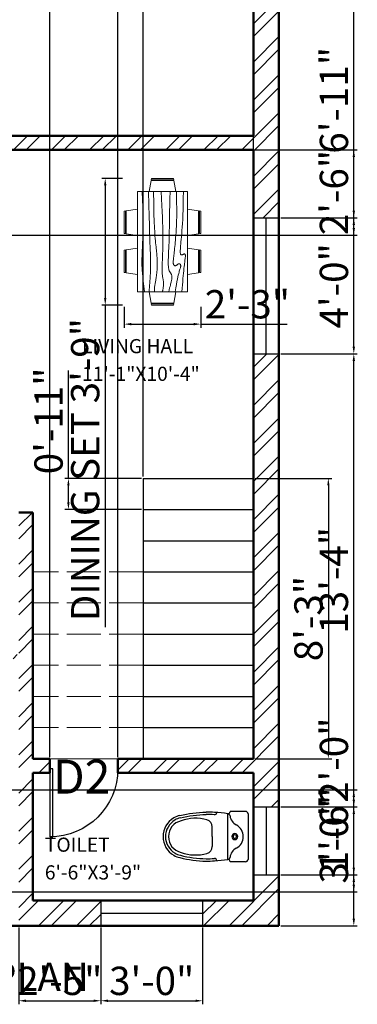
# Model space of a CAD drawing. Units: inches. Extents: x 3824 to 4289, y 1731 to 2259.
# Tile 4 of 5: x 4069 to 4188, y 1731 to 2079. Entities that reach past the tile are written whole.
import ezdxf

# ---------------------------------------------------------------- set-up
doc = ezdxf.new("R2010")
doc.units = ezdxf.units.IN
doc.linetypes.add('ACAD_ISO02W100', pattern=[15, 12, -3])
for name, color, linetype, lineweight in [('A-ANNO-DIMS', 2, 'Continuous', 18), ('A-ANNO-TEXT', 2, 'Continuous', 18), ('A-ANNO-TITL', 2, 'Continuous', 25), ('A-AREA-IDEN', 2, 'Continuous', 18), ('A-FLOR-FIXT', 9, 'Continuous', 18), ('A-FLOR-STRS-OVHD', 230, 'ACAD_ISO02W100', 18), ('A-FLOR-THRS', 8, 'Continuous', 18), ('A-FURN', 9, 'Continuous', 18), ('DOOR', 6, 'Continuous', 25), ('STAIRS', 230, 'Continuous', 25), ('WALL', 20, 'Continuous', 50), ('WINDOW', 4, 'Continuous', 25)]:
    doc.layers.add(name, color=color, linetype=linetype, lineweight=lineweight)
doc.layers.add('A-WALL-PATT', color=251, linetype='Continuous', lineweight=13, true_color=0x636466)
doc.layers.add('THIET-BI', color=21, linetype='Continuous')
doc.styles.get("Standard").update_dxf_attribs({"font": 'arial.ttf'})
doc.dimstyles.new('ISO-25', dxfattribs={"dimtxt": 10, "dimasz": 2.5, "dimexe": 1.25, "dimexo": 0.625, "dimtad": 1, "dimdec": 1, "dimlunit": 3, "dimtxsty": 'Standard', "dimcen": 2.5, "dimadec": 0, "dimazin": 0, "dimtfac": 1, "dimtdec": 1, "dimtmove": 0, "dimatfit": 3, "dimfxl": 1, "dimarcsym": 0})

# ---------------------------------------------------------------- blocks, each defined once
blk = doc.blocks.new('*U2')
for p, q in [((0, 0), (0, -6)), ((40, 0), (40, -6))]:
    blk.add_line(p, q)
blk.add_lwpolyline([(0, 0), (0, 40), (1.75, 40), (1.75, 0)], close=True)
blk.add_arc((0, 0), 40, 0, 90)
blk = doc.blocks.new('Dining Set - 36 x 72 in.')
for p, q in [((-22.2343, 26.00059), (-23.4847, 17.99762)), ((-22.2304, 26), (-5.7608, 26)), ((-22, 27.5), (-22.1562, 26.50042)), ((-5.8416, 26.5), (-22.1534, 26.5)), ((-22, 27.5), (-6, 27.5)), ((-5.8437, 26.49966), (-6, 27.5)), ((-4.5152, 17.99762), (-5.7655, 25.99926)), ((5.7657, 26.00059), (4.5153, 17.99762)), ((5.7696, 26), (22.2392, 26)), ((6, 27.5), (5.8438, 26.50042)), ((22.1584, 26.5), (5.8466, 26.5)), ((6, 27.5), (22, 27.5)), ((22.1563, 26.49966), (22, 27.5)), ((23.4848, 17.99762), (22.2345, 25.99926)), ((36, 18), (-36, 18)), ((-36, 18), (-36, -18)), ((36, -18), (36, 18)), ((-45.5, 8), (-44.5004, 8.15617)), ((-45.5, 8), (-45.5, -8)), ((-44.5, -8.15843), (-44.5, 8.15338)), ((-44.0006, 8.23428), (-35.9976, 9.48474)), ((-44, 8.23041), (-44, -8.23915)), ((44.0006, 8.23428), (35.9976, 9.48474)), ((44, 8.23041), (44, -8.23915)), ((44.5, -8.15843), (44.5, 8.15338)), ((45.5, 8), (44.5005, 8.15617)), ((45.5, 8), (45.5, -8)), ((-44.4997, -8.15631), (-45.5, -8)), ((-35.9976, -9.48476), (-43.9993, -8.2345)), ((35.9976, -9.48476), (43.9993, -8.2345)), ((44.4997, -8.15631), (45.5, -8)), ((-36, -18), (36, -18)), ((-22.2343, -26.0006), (-23.4847, -17.99762)), ((-4.5152, -17.99762), (-5.7655, -25.99928)), ((5.7657, -26.0006), (4.5153, -17.99762)), ((23.4848, -17.99762), (22.2345, -25.99928)), ((-22.2304, -26), (-5.7608, -26)), ((-22, -27.5), (-22.1562, -26.50044)), ((-5.8416, -26.5), (-22.1534, -26.5)), ((-22, -27.5), (-6, -27.5)), ((-5.8437, -26.49967), (-6, -27.5)), ((5.7696, -26), (22.2392, -26)), ((6, -27.5), (5.8438, -26.50044)), ((22.1584, -26.5), (5.8466, -26.5)), ((6, -27.5), (22, -27.5)), ((22.1563, -26.49967), (22, -27.5))]:
    blk.add_line(p, q)
for points in [[(-36, 15), (-31.1772, 14.97754), (-26.8079, 14.91406), (-22.8538, 14.81543), (-19.276, 14.6875), (-16.0362, 14.53613), (-13.0957, 14.36718), (-10.4159, 14.18652), (-7.9583, 14), (-5.6904, 13.81315), (-3.6035, 13.63021), (-1.6954, 13.45508), (0.0365, 13.29166), (1.5945, 13.14388), (2.9811, 13.01562), (4.1988, 12.9108), (5.25, 12.83333), (6.1393, 12.78613), (6.8802, 12.76823), (7.4883, 12.77767), (7.9792, 12.8125), (8.3685, 12.87077), (8.6719, 12.95052), (8.9049, 13.0498), (9.0833, 13.16666), (9.2205, 13.29899), (9.3216, 13.44401), (9.3895, 13.59879), (9.4271, 13.76041), (9.4373, 13.92594), (9.4232, 14.09245), (9.3875, 14.257), (9.3333, 14.41666), (9.2638, 14.56917), (9.1836, 14.71484), (9.0975, 14.85465), (9.0104, 14.98958), (8.9272, 15.1206), (8.8529, 15.2487), (8.7922, 15.37483), (8.75, 15.5), (8.7305, 15.62467), (8.7344, 15.74739), (8.7617, 15.86621), (8.8125, 15.97916), (8.8867, 16.08431), (8.9844, 16.17968), (9.1055, 16.26334), (9.25, 16.33333), (9.4189, 16.38802), (9.6172, 16.42708), (9.8506, 16.45052), (10.125, 16.45833), (10.4463, 16.45052), (10.8203, 16.42708), (11.2529, 16.38802), (11.75, 16.33333), (12.3184, 16.26318), (12.9694, 16.17838), (13.7151, 16.07991), (14.5677, 15.96875), (15.5395, 15.84586), (16.6426, 15.71224), (17.8893, 15.56884), (19.2917, 15.41666), (20.859, 15.25667), (22.5879, 15.08984), (24.4721, 14.91715), (26.5052, 14.73958), (28.6809, 14.5581), (30.9929, 14.3737), (33.4347, 14.18733), (36, 14)], [(-36, 10), (-28.9766, 10.14274), (-23.1725, 10.20442), (-18.4241, 10.19775), (-14.5677, 10.13541), (-11.4399, 10.03011), (-8.877, 9.89453), (-6.7154, 9.74137), (-4.7917, 9.58333), (-2.9698, 9.43082), (-1.2246, 9.28515), (0.4415, 9.14534), (2.026, 9.01041), (3.5266, 8.87939), (4.9408, 8.7513), (6.266, 8.62516), (7.5, 8.5), (8.6411, 8.37549), (9.6914, 8.2539), (10.6538, 8.13818), (11.5312, 8.03125), (12.3267, 7.93603), (13.043, 7.85547), (13.6831, 7.79248), (14.25, 7.75), (14.7471, 7.7303), (15.1797, 7.73307), (15.5537, 7.75732), (15.875, 7.80208), (16.1494, 7.86637), (16.3828, 7.94922), (16.5811, 8.04964), (16.75, 8.16666), (16.8944, 8.29915), (17.0143, 8.44531), (17.1089, 8.60319), (17.1771, 8.77083), (17.218, 8.94629), (17.2305, 9.1276), (17.2137, 9.31282), (17.1667, 9.5), (17.0895, 9.6875), (16.987, 9.875), (16.8649, 10.0625), (16.7292, 10.25), (16.5856, 10.4375), (16.4401, 10.625), (16.2985, 10.8125), (16.1667, 11), (16.05, 11.18733), (15.9518, 11.3737), (15.8752, 11.5581), (15.8229, 11.73958), (15.798, 11.91715), (15.8034, 12.08984), (15.842, 12.25667), (15.9167, 12.41666), (16.0295, 12.56836), (16.1784, 12.70833), (16.3605, 12.83268), (16.5729, 12.9375), (16.8127, 13.01888), (17.0768, 13.07291), (17.3625, 13.0957), (17.6667, 13.08333), (17.9894, 13.03312), (18.3418, 12.94726), (18.7382, 12.82918), (19.1927, 12.68229), (19.7195, 12.51001), (20.3327, 12.31575), (21.0465, 12.10294), (21.875, 11.875), (22.8357, 11.63354), (23.959, 11.37304), (25.2786, 11.08618), (26.8282, 10.76562), (28.6414, 10.40405), (30.752, 9.99414), (33.1936, 9.52856), (36, 9)], [(-36, 5.5), (-30.7157, 5.3348), (-26.069, 5.20963), (-21.9946, 5.11767), (-18.4271, 5.05208), (-15.3009, 5.00602), (-12.5508, 4.97265), (-10.1112, 4.94515), (-7.9167, 4.91666), (-5.909, 4.88167), (-4.0586, 4.83984), (-2.3429, 4.79215), (-0.7396, 4.73958), (0.7739, 4.6831), (2.22, 4.6237), (3.6213, 4.56233), (5, 4.5), (6.373, 4.43782), (7.7344, 4.3776), (9.0723, 4.32129), (10.375, 4.27083), (11.6309, 4.22819), (12.8281, 4.19531), (13.9551, 4.17415), (15, 4.16666), (15.954, 4.17448), (16.819, 4.19791), (17.6001, 4.23698), (18.3021, 4.29166), (18.9299, 4.36198), (19.4883, 4.44791), (19.9823, 4.54948), (20.4167, 4.66666), (20.7969, 4.79899), (21.1302, 4.94401), (21.4245, 5.09879), (21.6875, 5.26041), (21.9271, 5.42594), (22.1511, 5.59245), (22.3672, 5.757), (22.5834, 5.91666), (22.8065, 6.06868), (23.0404, 6.21093), (23.2879, 6.34147), (23.5521, 6.45833), (23.8358, 6.55957), (24.142, 6.64323), (24.4735, 6.70735), (24.8334, 6.75), (25.2235, 6.76969), (25.642, 6.76692), (26.0858, 6.74267), (26.5521, 6.69791), (27.0379, 6.63362), (27.5404, 6.55078), (28.0565, 6.45036), (28.5834, 6.33333), (29.1242, 6.19987), (29.7071, 6.04687), (30.3661, 5.87044), (31.1354, 5.66666), (32.0493, 5.43164), (33.142, 5.16146), (34.4475, 4.85221), (36, 4.5)], [(-36, -1), (-30.7915, -0.6591), (-26.0195, -0.38216), (-21.6519, -0.16284), (-17.6563, 0.00521), (-14.0005, 0.12833), (-10.6523, 0.21289), (-7.5796, 0.26522), (-4.75, 0.29166), (-2.134, 0.29793), (0.2878, 0.28711), (2.5317, 0.26163), (4.6146, 0.22396), (6.5529, 0.17651), (8.3633, 0.12174), (10.0623, 0.06209), (11.6667, 0), (13.1899, -0.06201), (14.6341, -0.1211), (15.9982, -0.17432), (17.2813, -0.21875), (18.4823, -0.25147), (19.6003, -0.26953), (20.6343, -0.27002), (21.5834, -0.25), (22.4481, -0.20768), (23.2357, -0.14584), (23.9549, -0.06836), (24.6146, 0.02083), (25.2235, 0.11784), (25.7904, 0.21875), (26.3241, 0.31966), (26.8334, 0.41666), (27.3265, 0.50618), (27.8099, 0.58593), (28.2894, 0.65397), (28.7709, 0.70833), (29.2601, 0.74707), (29.763, 0.76823), (30.2855, 0.76985), (30.8334, 0.75), (31.4088, 0.70784), (31.9994, 0.64713), (32.589, 0.57275), (33.1615, 0.48958), (33.7008, 0.4025), (34.1908, 0.3164), (34.6153, 0.23616), (34.9584, 0.16666), (35.2099, 0.11165), (35.3848, 0.07031), (35.504, 0.04069), (35.5886, 0.02083), (35.6594, 0.00879), (35.7377, 0.0026), (35.8442, 0.00032), (36, 0)], [(-36, -6.5), (-27.1843, -6.31267), (-20.084, -6.1263), (-14.469, -5.9419), (-10.1094, -5.76042), (-6.7752, -5.58285), (-4.2363, -5.41016), (-2.2629, -5.24333), (-0.625, -5.08334), (0.8708, -4.93099), (2.2715, -4.78646), (3.5872, -4.64974), (4.8281, -4.52084), (6.0046, -4.39974), (7.127, -4.28646), (8.2053, -4.18099), (9.25, -4.08334), (10.2705, -3.99382), (11.2734, -3.91407), (12.2647, -3.84603), (13.25, -3.79167), (14.2354, -3.75293), (15.2266, -3.73177), (16.2295, -3.73015), (17.25, -3.75), (18.2912, -3.79248), (19.3451, -3.85547), (20.4009, -3.93604), (21.4479, -4.03125), (22.4754, -4.13819), (23.4727, -4.25391), (24.4289, -4.37549), (25.3334, -4.5), (26.1785, -4.62492), (26.9694, -4.74935), (27.7145, -4.87281), (28.4219, -4.99479), (29.1, -5.11483), (29.7572, -5.23242), (30.4016, -5.34709), (31.0417, -5.45834), (31.6837, -5.56437), (32.3262, -5.65821), (32.9658, -5.73153), (33.599, -5.77604), (34.2224, -5.78345), (34.8327, -5.74545), (35.4264, -5.65373), (36, -5.5)], [(-36, -10), (-26.4022, -9.81299), (-18.4675, -9.62891), (-11.9839, -9.45069), (-6.7396, -9.28125), (-2.5226, -9.12354), (0.8789, -8.98047), (3.6769, -8.85498), (6.0833, -8.75), (8.2767, -8.66765), (10.3021, -8.60677), (12.1712, -8.56543), (13.8958, -8.54167), (15.4876, -8.53353), (16.9583, -8.53907), (18.3197, -8.55632), (19.5834, -8.58334), (20.7616, -8.61841), (21.8685, -8.66081), (22.9188, -8.71004), (23.9271, -8.76563), (24.9081, -8.82707), (25.8763, -8.89388), (26.8465, -8.96558), (27.8334, -9.04167), (28.8474, -9.12118), (29.8828, -9.20117), (30.93, -9.27824), (31.9792, -9.34896), (33.0205, -9.40991), (34.0443, -9.45768), (35.0407, -9.48885), (36, -9.5)], [(-36, -14.5), (-30.0881, -14.33513), (-25.0332, -14.21224), (-20.7312, -14.12647), (-17.0781, -14.07292), (-13.97, -14.04671), (-11.3027, -14.04297), (-8.9724, -14.05681), (-6.875, -14.08334), (-4.9224, -14.11833), (-3.0905, -14.16016), (-1.3709, -14.20785), (0.2448, -14.26042), (1.7647, -14.3169), (3.1973, -14.3763), (4.5507, -14.43767), (5.8333, -14.5), (7.0554, -14.5621), (8.235, -14.62175), (9.3922, -14.67652), (10.5469, -14.72396), (11.7192, -14.76164), (12.929, -14.78711), (14.1965, -14.79794), (15.5417, -14.79167), (16.9933, -14.76424), (18.6152, -14.70508), (20.4804, -14.60197), (22.6615, -14.44271), (25.2312, -14.21509), (28.2624, -13.9069), (31.8277, -13.50594), (36, -13)]]:
    blk.add_lwpolyline(points)
blk = doc.blocks.new('A$C7C314EA1')
at = {"layer": 'THIET-BI'}
for p, q in [((20, 420), (150, 420)), ((0, 20), (0, 400)), ((170, 400), (170, 20)), ((300, 210), (300, 292.2)), ((300, 210), (300, 127.8)), ((20, 0), (150, 0)), ((20, 0), (150, 0))]:
    blk.add_line(p, q, dxfattribs=at)
for points in [[(279.9, 412.5, 0.02753), (170, 400, 0.02753)], [(569.7, 385.6, 0.054905), (350, 415, 0.054905)], [(564.9, 366.1, 0.054905), (349.5, 395, 0.054905)], [(300, 210), (300, 290, 0.704392)], [(300, 210), (300, 130, -0.704392)], [(170, 20, 0.02753), (279.9, 7.5, 0.02753)], [(564.9, 53.9, -0.054905), (349.5, 25, -0.054905)], [(569.7, 34.4, -0.054905), (350, 5, -0.054905)]]:
    blk.add_lwpolyline(points, format="xyb", dxfattribs=at)
for centre, radius, start, end in [((20, 400), 20, 90, 180), ((170, 420), 20, 180, 270), ((279.9, 412.5), 20, 184.59048, 273.88227), ((350, -585), 1000, 90, 94.02044), ((51, 395.2), 100, 298.13818, 352.73228), ((170, 380), 20, 90, 172.73228), ((350, -585), 980, 90, 94.02044), ((360, 292.2), 60, 105.92494, 180), ((439, 15.2), 348.1, 69.70099, 105.92494), ((530, 210), 135, 0, 77.24247), ((530, 210), 160, 60, 77.24247), ((530, 210), 180, 60, 77.24247), ((530, 210), 160, 0, 60), ((530, 210), 180, 0, 60), ((150, 210), 110, 118.13818, 180), ((150, 210), 110, 180, 241.86182), ((150, 210), 110, 180, 241.86182), ((110, 210), 25, 0, 180), ((110, 210), 25, 0, 180), ((110, 210), 25, 180, 0), ((110, 210), 25, 180, 0), ((110, 210), 15, 0, 180), ((110, 210), 15, 0, 180), ((110, 210), 15, 180, 0), ((110, 210), 15, 180, 0), ((530, 210), 135, 282.75753, 0), ((530, 210), 160, 300, 0), ((530, 210), 180, 300, 0), ((51, 24.8), 100, 7.26772, 61.86182), ((51, 24.8), 100, 7.26772, 61.86182), ((360, 127.8), 60, 180, 254.07506), ((20, 20), 20, 180, 270), ((170, 0), 20, 90, 180), ((170, 40), 20, 187.26772, 270), ((170, 40), 20, 187.26772, 270), ((279.9, 7.5), 20, 86.11773, 175.40952), ((350, 1005), 1000, 265.97956, 270), ((350, 1005), 980, 265.97956, 270), ((439, 404.8), 348.1, 254.07506, 290.29901), ((530, 210), 160, 282.75753, 300), ((530, 210), 180, 282.75753, 300)]:
    blk.add_arc(centre, radius, start, end, dxfattribs=at)
blk = doc.blocks.new('*D20')
at = {"layer": 'A-ANNO-DIMS', "color": 0, "lineweight": -2, "transparency": 16777216}
for p, q in [((4105.21, 2022.56), (4097.87, 2022.56)), ((4099.12, 2020.06), (4099.12, 1980.29)), ((4105.21, 1977.79), (4097.87, 1977.79)), ((4099.12, 1977.79), (4099.12, 1864.13))]:
    blk.add_line(p, q, dxfattribs=at)
at = {"layer": 'A-ANNO-DIMS', "color": 0, "transparency": 16777216}
for points in [[(4098.7, 2020.06), (4099.53, 2020.06), (4099.12, 2022.56)], [(4098.7, 1980.29), (4099.53, 1980.29), (4099.12, 1977.79)]]:
    blk.add_solid(points, dxfattribs=at)
at = {"layer": 'Defpoints', "color": 0, "transparency": 16777216}
for p in [(4105.83, 2022.56), (4099.12, 1977.79), (4105.83, 1977.79)]:
    blk.add_point(p, dxfattribs=at)
at = {"layer": 'A-ANNO-DIMS', "color": 0, "transparency": 16777216, "insert": (4093.32, 1919.71), "char_height": 10, "attachment_point": 5, "rotation": 90}
blk.add_mtext('DINING SET 3\'-9"', dxfattribs=at)
blk = doc.blocks.new('*D21')
at = {"layer": 'A-ANNO-DIMS', "color": 0, "lineweight": -2, "transparency": 16777216}
for p, q in [((4105.83, 1977.17), (4105.83, 1969.83)), ((4132.89, 1977.17), (4132.89, 1969.83)), ((4108.33, 1971.08), (4130.39, 1971.08)), ((4132.89, 1971.08), (4163.39, 1971.08))]:
    blk.add_line(p, q, dxfattribs=at)
at = {"layer": 'A-ANNO-DIMS', "color": 0, "transparency": 16777216}
for points in [[(4108.33, 1971.5), (4108.33, 1970.66), (4105.83, 1971.08)], [(4130.39, 1971.5), (4130.39, 1970.66), (4132.89, 1971.08)]]:
    blk.add_solid(points, dxfattribs=at)
at = {"layer": 'Defpoints', "color": 0, "transparency": 16777216}
for p in [(4105.83, 1977.79), (4132.89, 1977.79), (4132.89, 1971.08)]:
    blk.add_point(p, dxfattribs=at)
at = {"layer": 'A-ANNO-DIMS', "color": 0, "transparency": 16777216, "insert": (4149.39, 1976.81), "char_height": 10, "attachment_point": 5}
blk.add_mtext('2\'-3"', dxfattribs=at)
blk = doc.blocks.new('*D32')
at = {"layer": 'A-ANNO-DIMS', "color": 0, "lineweight": -2, "transparency": 16777216}
for p, q in [((4187, 1776.62), (4187, 1806.01)), ((4161.18, 1776.62), (4188.25, 1776.62)), ((4187, 1761.12), (4187, 1774.12)), ((4161.18, 1758.62), (4188.25, 1758.62))]:
    blk.add_line(p, q, dxfattribs=at)
at = {"layer": 'A-ANNO-DIMS', "color": 0, "transparency": 16777216}
for points in [[(4186.59, 1774.12), (4187.42, 1774.12), (4187, 1776.62)], [(4186.59, 1761.12), (4187.42, 1761.12), (4187, 1758.62)]]:
    blk.add_solid(points, dxfattribs=at)
at = {"layer": 'Defpoints', "color": 0, "transparency": 16777216}
for p in [(4160.55, 1776.62), (4187, 1776.62), (4160.55, 1758.62)]:
    blk.add_point(p, dxfattribs=at)
at = {"layer": 'A-ANNO-DIMS', "color": 0, "transparency": 16777216, "insert": (4181.27, 1792.56), "char_height": 10, "attachment_point": 5, "rotation": 90}
blk.add_mtext('1\'-6"', dxfattribs=at)
blk = doc.blocks.new('*D33')
at = {"layer": 'A-ANNO-DIMS', "color": 0, "lineweight": -2, "transparency": 16777216}
for p, q in [((4187, 1800.62), (4187, 1831.12)), ((4161.18, 1800.62), (4188.25, 1800.62)), ((4187, 1779.12), (4187, 1798.12)), ((4161.18, 1776.62), (4188.25, 1776.62))]:
    blk.add_line(p, q, dxfattribs=at)
at = {"layer": 'A-ANNO-DIMS', "color": 0, "transparency": 16777216}
for points in [[(4186.59, 1798.12), (4187.42, 1798.12), (4187, 1800.62)], [(4186.59, 1779.12), (4187.42, 1779.12), (4187, 1776.62)]]:
    blk.add_solid(points, dxfattribs=at)
at = {"layer": 'Defpoints', "color": 0, "transparency": 16777216}
for p in [(4160.55, 1800.62), (4187, 1800.62), (4160.55, 1776.62)]:
    blk.add_point(p, dxfattribs=at)
at = {"layer": 'A-ANNO-DIMS', "color": 0, "transparency": 16777216, "insert": (4181.27, 1817.12), "char_height": 10, "attachment_point": 5, "rotation": 90}
blk.add_mtext('2\'-0"', dxfattribs=at)
blk = doc.blocks.new('*D34')
at = {"layer": 'A-ANNO-DIMS', "color": 0, "lineweight": -2, "transparency": 16777216}
for p, q in [((4161.18, 1960.62), (4188.25, 1960.62)), ((4187, 1803.12), (4187, 1958.12)), ((4161.18, 1800.62), (4188.25, 1800.62))]:
    blk.add_line(p, q, dxfattribs=at)
at = {"layer": 'A-ANNO-DIMS', "color": 0, "transparency": 16777216}
for points in [[(4186.59, 1958.12), (4187.42, 1958.12), (4187, 1960.62)], [(4186.59, 1803.12), (4187.42, 1803.12), (4187, 1800.62)]]:
    blk.add_solid(points, dxfattribs=at)
at = {"layer": 'Defpoints', "color": 0, "transparency": 16777216}
for p in [(4160.55, 1960.62), (4187, 1960.62), (4160.55, 1800.62)]:
    blk.add_point(p, dxfattribs=at)
at = {"layer": 'A-ANNO-DIMS', "color": 0, "transparency": 16777216, "insert": (4181.27, 1880.62), "char_height": 10, "attachment_point": 5, "rotation": 90}
blk.add_mtext('13\'-4"', dxfattribs=at)
blk = doc.blocks.new('*D35')
at = {"layer": 'A-ANNO-DIMS', "color": 0, "lineweight": -2, "transparency": 16777216}
for p, q in [((4161.18, 2008.62), (4188.25, 2008.62)), ((4187, 1963.12), (4187, 2006.12)), ((4161.18, 1960.62), (4188.25, 1960.62))]:
    blk.add_line(p, q, dxfattribs=at)
at = {"layer": 'A-ANNO-DIMS', "color": 0, "transparency": 16777216}
for points in [[(4186.59, 2006.12), (4187.42, 2006.12), (4187, 2008.62)], [(4186.59, 1963.12), (4187.42, 1963.12), (4187, 1960.62)]]:
    blk.add_solid(points, dxfattribs=at)
at = {"layer": 'Defpoints', "color": 0, "transparency": 16777216}
for p in [(4160.55, 2008.62), (4187, 2008.62), (4160.55, 1960.62)]:
    blk.add_point(p, dxfattribs=at)
at = {"layer": 'A-ANNO-DIMS', "color": 0, "transparency": 16777216, "insert": (4181.27, 1984.62), "char_height": 10, "attachment_point": 5, "rotation": 90}
blk.add_mtext('4\'-0"', dxfattribs=at)
blk = doc.blocks.new('*D36')
at = {"layer": 'A-ANNO-DIMS', "color": 0, "lineweight": -2, "transparency": 16777216}
for p, q in [((4161.18, 2091.62), (4188.25, 2091.62)), ((4187, 2011.12), (4187, 2089.12)), ((4161.18, 2008.62), (4188.25, 2008.62))]:
    blk.add_line(p, q, dxfattribs=at)
at = {"layer": 'A-ANNO-DIMS', "color": 0, "transparency": 16777216}
for points in [[(4186.59, 2089.12), (4187.42, 2089.12), (4187, 2091.62)], [(4186.59, 2011.12), (4187.42, 2011.12), (4187, 2008.62)]]:
    blk.add_solid(points, dxfattribs=at)
at = {"layer": 'Defpoints', "color": 0, "transparency": 16777216}
for p in [(4160.55, 2091.62), (4187, 2091.62), (4160.55, 2008.62)]:
    blk.add_point(p, dxfattribs=at)
at = {"layer": 'A-ANNO-DIMS', "color": 0, "transparency": 16777216, "insert": (4181.27, 2050.12), "char_height": 10, "attachment_point": 5, "rotation": 90}
blk.add_mtext('6\'-11"', dxfattribs=at)
blk = doc.blocks.new('*D40')
at = {"layer": 'A-ANNO-DIMS', "color": 0, "lineweight": -2, "transparency": 16777216}
for p, q in [((4068.55, 1757.99), (4068.55, 1730.92)), ((4097.55, 1757.99), (4097.55, 1730.92)), ((4071.05, 1732.17), (4095.05, 1732.17))]:
    blk.add_line(p, q, dxfattribs=at)
at = {"layer": 'A-ANNO-DIMS', "color": 0, "transparency": 16777216}
for points in [[(4071.05, 1732.59), (4071.05, 1731.75), (4068.55, 1732.17)], [(4095.05, 1732.59), (4095.05, 1731.75), (4097.55, 1732.17)]]:
    blk.add_solid(points, dxfattribs=at)
at = {"layer": 'Defpoints', "color": 0, "transparency": 16777216}
for p in [(4068.55, 1758.62), (4097.55, 1758.62), (4097.55, 1732.17)]:
    blk.add_point(p, dxfattribs=at)
at = {"layer": 'A-ANNO-DIMS', "color": 0, "transparency": 16777216, "insert": (4083.05, 1737.9), "char_height": 10, "attachment_point": 5}
blk.add_mtext('2\'-5"', dxfattribs=at)
blk = doc.blocks.new('*D41')
at = {"layer": 'A-ANNO-DIMS', "color": 0, "lineweight": -2, "transparency": 16777216}
for p, q in [((4097.55, 1757.99), (4097.55, 1730.92)), ((4133.55, 1757.99), (4133.55, 1730.92)), ((4100.05, 1732.17), (4131.05, 1732.17))]:
    blk.add_line(p, q, dxfattribs=at)
at = {"layer": 'A-ANNO-DIMS', "color": 0, "transparency": 16777216}
for points in [[(4100.05, 1732.59), (4100.05, 1731.75), (4097.55, 1732.17)], [(4131.05, 1732.59), (4131.05, 1731.75), (4133.55, 1732.17)]]:
    blk.add_solid(points, dxfattribs=at)
at = {"layer": 'Defpoints', "color": 0, "transparency": 16777216}
for p in [(4097.55, 1758.62), (4133.55, 1758.62), (4133.55, 1732.17)]:
    blk.add_point(p, dxfattribs=at)
at = {"layer": 'A-ANNO-DIMS', "color": 0, "transparency": 16777216, "insert": (4115.55, 1737.9), "char_height": 10, "attachment_point": 5}
blk.add_mtext('3\'-0"', dxfattribs=at)
blk = doc.blocks.new('*D49')
at = {"layer": 'A-ANNO-DIMS', "color": 0, "lineweight": -2, "transparency": 16777216}
for p, q in [((3965.18, 1806.62), (4188.25, 1806.62)), ((4187, 1773.12), (4187, 1804.12)), ((3965.18, 1770.62), (4188.25, 1770.62))]:
    blk.add_line(p, q, dxfattribs=at)
at = {"layer": 'A-ANNO-DIMS', "color": 0, "transparency": 16777216}
for points in [[(4186.59, 1804.12), (4187.42, 1804.12), (4187, 1806.62)], [(4186.59, 1773.12), (4187.42, 1773.12), (4187, 1770.62)]]:
    blk.add_solid(points, dxfattribs=at)
at = {"layer": 'Defpoints', "color": 0, "transparency": 16777216}
for p in [(3964.55, 1806.62), (4187, 1806.62), (3964.55, 1770.62)]:
    blk.add_point(p, dxfattribs=at)
at = {"layer": 'A-ANNO-DIMS', "color": 0, "transparency": 16777216, "insert": (4181.27, 1788.62), "char_height": 10, "attachment_point": 5, "rotation": 90}
blk.add_mtext('3\'-0"', dxfattribs=at)
blk = doc.blocks.new('*D50')
at = {"layer": 'A-ANNO-DIMS', "color": 0, "lineweight": -2, "transparency": 16777216}
for p, q in [((4079.55, 1818.24), (4079.55, 2230.32)), ((4082.05, 2229.07), (4101.05, 2229.07)), ((4103.55, 1818.24), (4103.55, 2230.32)), ((4103.55, 2229.07), (4134.06, 2229.07))]:
    blk.add_line(p, q, dxfattribs=at)
at = {"layer": 'A-ANNO-DIMS', "color": 0, "transparency": 16777216}
for points in [[(4082.05, 2229.49), (4082.05, 2228.65), (4079.55, 2229.07)], [(4101.05, 2229.49), (4101.05, 2228.65), (4103.55, 2229.07)]]:
    blk.add_solid(points, dxfattribs=at)
at = {"layer": 'Defpoints', "color": 0, "transparency": 16777216}
for p in [(4103.55, 2229.07), (4079.55, 1817.62), (4103.55, 1817.62)]:
    blk.add_point(p, dxfattribs=at)
at = {"layer": 'A-ANNO-DIMS', "color": 0, "transparency": 16777216, "insert": (4120.05, 2234.8), "char_height": 10, "attachment_point": 5}
blk.add_mtext('2\'-0"', dxfattribs=at)
blk = doc.blocks.new('*D51')
at = {"layer": 'A-ANNO-DIMS', "color": 0, "lineweight": -2, "transparency": 16777216}
for p, q in [((4112.55, 1917.24), (4112.55, 2230.32)), ((4115.05, 2229.07), (4149.05, 2229.07)), ((4151.55, 1917.24), (4151.55, 2230.32))]:
    blk.add_line(p, q, dxfattribs=at)
at = {"layer": 'A-ANNO-DIMS', "color": 0, "transparency": 16777216}
for points in [[(4115.05, 2229.49), (4115.05, 2228.65), (4112.55, 2229.07)], [(4149.05, 2229.49), (4149.05, 2228.65), (4151.55, 2229.07)]]:
    blk.add_solid(points, dxfattribs=at)
at = {"layer": 'Defpoints', "color": 0, "transparency": 16777216}
for p in [(4151.55, 2229.07), (4112.55, 1916.62), (4151.55, 1916.62)]:
    blk.add_point(p, dxfattribs=at)
at = {"layer": 'A-ANNO-DIMS', "color": 0, "transparency": 16777216, "insert": (4132.05, 2234.8), "char_height": 10, "attachment_point": 5}
blk.add_mtext('3\'-3"', dxfattribs=at)
blk = doc.blocks.new('*D52')
at = {"layer": 'A-ANNO-DIMS', "color": 0, "lineweight": -2, "transparency": 16777216}
for p, q in [((4152.18, 1916.62), (4179.25, 1916.62)), ((4178, 1914.12), (4178, 1820.12)), ((4152.18, 1817.62), (4179.25, 1817.62))]:
    blk.add_line(p, q, dxfattribs=at)
at = {"layer": 'A-ANNO-DIMS', "color": 0, "transparency": 16777216}
for points in [[(4177.59, 1914.12), (4178.42, 1914.12), (4178, 1916.62)], [(4177.59, 1820.12), (4178.42, 1820.12), (4178, 1817.62)]]:
    blk.add_solid(points, dxfattribs=at)
at = {"layer": 'Defpoints', "color": 0, "transparency": 16777216}
for p in [(4151.55, 1916.62), (4151.55, 1817.62), (4178, 1817.62)]:
    blk.add_point(p, dxfattribs=at)
at = {"layer": 'A-ANNO-DIMS', "color": 0, "transparency": 16777216, "insert": (4172.27, 1867.12), "char_height": 10, "attachment_point": 5, "rotation": 90}
blk.add_mtext('8\'-3"', dxfattribs=at)
blk = doc.blocks.new('*D53')
at = {"layer": 'A-ANNO-DIMS', "color": 0, "lineweight": -2, "transparency": 16777216}
for p, q in [((4086.1, 1916.62), (4086.1, 1954.72)), ((4111.93, 1916.62), (4084.85, 1916.62)), ((4086.1, 1908.12), (4086.1, 1914.12)), ((4111.93, 1905.62), (4084.85, 1905.62))]:
    blk.add_line(p, q, dxfattribs=at)
at = {"layer": 'A-ANNO-DIMS', "color": 0, "transparency": 16777216}
for points in [[(4085.69, 1914.12), (4086.52, 1914.12), (4086.1, 1916.62)], [(4085.69, 1908.12), (4086.52, 1908.12), (4086.1, 1905.62)]]:
    blk.add_solid(points, dxfattribs=at)
at = {"layer": 'Defpoints', "color": 0, "transparency": 16777216}
for p in [(4086.1, 1916.62), (4112.55, 1916.62), (4112.55, 1905.62)]:
    blk.add_point(p, dxfattribs=at)
at = {"layer": 'A-ANNO-DIMS', "color": 0, "transparency": 16777216, "insert": (4080.37, 1936.92), "char_height": 10, "attachment_point": 5, "rotation": 90}
blk.add_mtext('0\'-11"', dxfattribs=at)
blk = doc.blocks.new('*D62')
at = {"layer": 'A-ANNO-DIMS', "color": 0, "lineweight": -2, "transparency": 16777216}
for p, q in [((3898.51, 2032.62), (4188.25, 2032.62)), ((4187, 2005), (4187, 2030.12)), ((3898.51, 2002.5), (4188.25, 2002.5))]:
    blk.add_line(p, q, dxfattribs=at)
at = {"layer": 'A-ANNO-DIMS', "color": 0, "transparency": 16777216}
for points in [[(4186.59, 2030.12), (4187.42, 2030.12), (4187, 2032.62)], [(4186.59, 2005), (4187.42, 2005), (4187, 2002.5)]]:
    blk.add_solid(points, dxfattribs=at)
at = {"layer": 'Defpoints', "color": 0, "transparency": 16777216}
for p in [(3897.89, 2032.62), (4187, 2032.62), (3897.89, 2002.5)]:
    blk.add_point(p, dxfattribs=at)
at = {"layer": 'A-ANNO-DIMS', "color": 0, "transparency": 16777216, "insert": (4181.27, 2017.56), "char_height": 10, "attachment_point": 5, "rotation": 90}
blk.add_mtext('2\'-6"', dxfattribs=at)

msp = doc.modelspace()

# ---------------------------------------------------------------- hatches: boundary and pattern name
at = {"layer": 'A-WALL-PATT'}
h = msp.add_hatch(dxfattribs=at)
h.set_pattern_fill('ANSI32', color=256)
h.paths.add_polyline_path([(4160.55, 2091.62), (4151.55, 2091.62), (4151.55, 2037.62), (4063.55, 2037.62), (4063.55, 2032.62), (4151.55, 2032.62), (4151.55, 2008.62), (4160.55, 2008.62)])
h = msp.add_hatch(dxfattribs=at)
h.set_pattern_fill('ANSI32', color=256)
h.paths.add_polyline_path([(4160.55, 1960.62), (4151.55, 1960.62), (4151.55, 1817.62), (4103.55, 1817.62), (4103.55, 1814.02), (4103.55, 1812.62), (4151.55, 1812.62), (4151.55, 1800.62), (4160.55, 1800.62)])
h = msp.add_hatch(dxfattribs=at)
h.set_pattern_fill('ANSI32', color=256)
h.paths.add_polyline_path([(4073.55, 1904.62), (4068.55, 1904.62), (4068.55, 1854.39), (4066.55, 1854.39), (4066.55, 1849.39), (4068.55, 1849.39), (4068.55, 1767.62), (4068.55, 1758.62), (4097.55, 1758.62), (4097.55, 1767.62), (4073.55, 1767.62), (4073.55, 1812.62), (4079.55, 1812.62), (4079.55, 1817.62), (4073.55, 1817.62)])
h = msp.add_hatch(dxfattribs=at)
h.set_pattern_fill('ANSI32', color=256)
h.paths.add_polyline_path([(4160.55, 1776.62), (4151.55, 1776.62), (4151.55, 1767.62), (4133.55, 1767.62), (4133.55, 1758.62), (4160.55, 1758.62)])

# ---------------------------------------------------------------- linework, layer by layer
at = {"layer": 'A-FLOR-STRS-OVHD'}
for p, q in [((4112.55, 1883.62), (4073.55, 1883.62)), ((4112.55, 1872.62), (4073.55, 1872.62)), ((4112.55, 1861.62), (4073.55, 1861.62)), ((4112.55, 1850.62), (4073.55, 1850.62)), ((4112.55, 1839.62), (4073.55, 1839.62)), ((4112.55, 1828.62), (4073.55, 1828.62))]:
    msp.add_line(p, q, dxfattribs=at)
at = {"layer": 'A-FLOR-THRS'}
msp.add_line((4079.55, 1817.62), (4103.55, 1817.62), dxfattribs=at)
at = {"layer": 'STAIRS'}
for p, q in [((4112.55, 1916.62), (4151.55, 1916.62)), ((4112.55, 1916.62), (4112.55, 1817.62)), ((4112.55, 1905.62), (4151.55, 1905.62)), ((4112.55, 1894.62), (4151.55, 1894.62)), ((4112.55, 1883.62), (4151.55, 1883.62)), ((4112.55, 1872.62), (4151.55, 1872.62)), ((4112.55, 1861.62), (4151.55, 1861.62)), ((4112.55, 1850.62), (4151.55, 1850.62)), ((4112.55, 1839.62), (4151.55, 1839.62)), ((4112.55, 1828.62), (4151.55, 1828.62))]:
    msp.add_line(p, q, dxfattribs=at)
at = {"layer": 'WALL'}
for p, q in [((4160.55, 2202.62), (4160.55, 1758.62)), ((4151.55, 2193.62), (4151.55, 2037.62)), ((4063.55, 2037.62), (4151.55, 2037.62)), ((4063.55, 2032.62), (4151.55, 2032.62)), ((4151.55, 2032.62), (4151.55, 1817.62)), ((4068.55, 1904.62), (4073.55, 1904.62)), ((4073.55, 1904.62), (4073.55, 1817.62)), ((4073.55, 1817.62), (4079.55, 1817.62)), ((4079.55, 1817.62), (4079.55, 1812.62)), ((4103.55, 1817.62), (4103.55, 1812.62)), ((4103.55, 1817.62), (4151.55, 1817.62)), ((4073.55, 1812.62), (4079.55, 1812.62)), ((4073.55, 1812.62), (4073.55, 1767.62)), ((4103.55, 1812.62), (4151.55, 1812.62)), ((4151.55, 1812.62), (4151.55, 1767.62)), ((4073.55, 1767.62), (4151.55, 1767.62)), ((4013.55, 1758.62), (4160.55, 1758.62))]:
    msp.add_line(p, q, dxfattribs=at)
at = {"layer": 'WINDOW'}
for p, q in [((4151.55, 2008.62), (4160.55, 2008.62)), ((4156.05, 1960.62), (4156.05, 2008.62)), ((4151.55, 1960.62), (4160.55, 1960.62)), ((4151.55, 1800.62), (4160.55, 1800.62)), ((4156.05, 1800.62), (4156.05, 1776.62)), ((4151.55, 1776.62), (4160.55, 1776.62)), ((4097.55, 1767.62), (4097.55, 1758.62)), ((4133.55, 1767.62), (4133.55, 1758.62)), ((4097.55, 1763.12), (4133.55, 1763.12))]:
    msp.add_line(p, q, dxfattribs=at)

# ---------------------------------------------------------------- block references
at = {"layer": 'A-FLOR-FIXT', "xscale": 0.042307961426094, "yscale": 0.042307961426094, "zscale": 0.042307961426094, "rotation": 180}
msp.add_blockref('A$C7C314EA1', (4149.6, 1799.02), dxfattribs=at)
at = {"layer": 'A-FURN', "xscale": 0.4919098676543778, "yscale": 0.4919098676543778, "zscale": 0.4919098676543778, "rotation": 270.0000000116096}
msp.add_blockref('Dining Set - 36 x 72 in.', (4119.36, 2000.18), dxfattribs=at)
at = {"layer": 'DOOR', "xscale": -0.6, "yscale": 0.6, "zscale": 0.6, "rotation": 180}
msp.add_blockref('*U2', (4079.55, 1814.02), dxfattribs=at)

# ---------------------------------------------------------------- texts
at = {"layer": 'A-ANNO-TEXT'}
msp.add_text('D2', height=12, dxfattribs=at).set_placement((4080.6, 1805.29))
at = {"layer": 'A-ANNO-TITL'}
msp.add_text('GROUND FLOOR PLAN', height=10, dxfattribs=at).set_placement((3951.87, 1735.58))
at = {"layer": 'A-AREA-IDEN'}
for s, p in [('LIVING HALL', (4090.91, 1960.82)), ('11\'-1"X10\'-4"', (4090.91, 1951.04)), ('TOILET', (4077.76, 1784.78)), ('6\'-6"X3\'-9"', (4077.76, 1774.99))]:
    msp.add_text(s, height=5, dxfattribs=at).set_placement(p)

# ---------------------------------------------------------------- dimensions: what is measured, and where the dimension line sits
at = {"layer": 'A-ANNO-DIMS'}
for base, p1, p2, picture, middle in [((4103.55, 2229.07), (4079.55, 1817.62), (4103.55, 1817.62), '*D50', (4120.05, 2234.8)), ((4151.55, 2229.07), (4112.55, 1916.62), (4151.55, 1916.62), '*D51', (4132.05, 2234.8)), ((4097.55, 1732.17), (4068.55, 1758.62), (4097.55, 1758.62), '*D40', (4083.05, 1737.9)), ((4133.55, 1732.17), (4097.55, 1758.62), (4133.55, 1758.62), '*D41', (4115.55, 1737.9))]:
    dim = msp.add_linear_dim(base=base, p1=p1, p2=p2, dimstyle='ISO-25', override={"dimdec": 1, "dimlfac": 1, "dimrnd": 0, "dimzin": 1, "dimdsep": 46, "dimlunit": 4, "dimfrac": 2}, dxfattribs=at)
    dim.commit()
    dim.dimension.update_dxf_attribs({"geometry": picture, "text_midpoint": middle})
for base, p1, p2, angle, picture, middle in [((4187, 2091.62), (4160.55, 2008.62), (4160.55, 2091.62), 90, '*D36', (4181.27, 2050.12)), ((4187, 2032.62), (3897.89, 2002.5), (3897.89, 2032.62), 90, '*D62', (4181.27, 2017.56)), ((4187, 2008.62), (4160.55, 1960.62), (4160.55, 2008.62), 90, '*D35', (4181.27, 1984.62)), ((4132.89, 1971.08), (4105.83, 1977.79), (4132.89, 1977.79), 0, '*D21', (4149.39, 1976.81)), ((4187, 1960.62), (4160.55, 1800.62), (4160.55, 1960.62), 90, '*D34', (4181.27, 1880.62)), ((4086.1, 1916.62), (4112.55, 1905.62), (4112.55, 1916.62), 90, '*D53', (4080.37, 1936.92)), ((4178, 1817.62), (4151.55, 1916.62), (4151.55, 1817.62), 270, '*D52', (4172.27, 1867.12)), ((4187, 1800.62), (4160.55, 1776.62), (4160.55, 1800.62), 90, '*D33', (4181.27, 1817.12)), ((4187, 1806.62), (3964.55, 1770.62), (3964.55, 1806.62), 90, '*D49', (4181.27, 1788.62)), ((4187, 1776.62), (4160.55, 1758.62), (4160.55, 1776.62), 90, '*D32', (4181.27, 1792.56))]:
    dim = msp.add_linear_dim(base=base, p1=p1, p2=p2, angle=angle, dimstyle='ISO-25', override={"dimdec": 1, "dimlfac": 1, "dimrnd": 0, "dimzin": 1, "dimdsep": 46, "dimlunit": 4, "dimfrac": 2}, dxfattribs=at)
    dim.commit()
    dim.dimension.update_dxf_attribs({"geometry": picture, "text_midpoint": middle})
dim = msp.add_linear_dim(base=(4099.12, 1977.79), p1=(4105.83, 2022.56), p2=(4105.83, 1977.79), angle=270, text='DINING SET <>', dimstyle='ISO-25', override={"dimdec": 1, "dimlfac": 1, "dimrnd": 0, "dimzin": 1, "dimdsep": 46, "dimlunit": 4, "dimfrac": 2}, dxfattribs=at)
dim.commit()
dim.dimension.update_dxf_attribs({"geometry": '*D20', "text_midpoint": (4093.32, 1919.71)})

doc.saveas('drawing.dxf')
